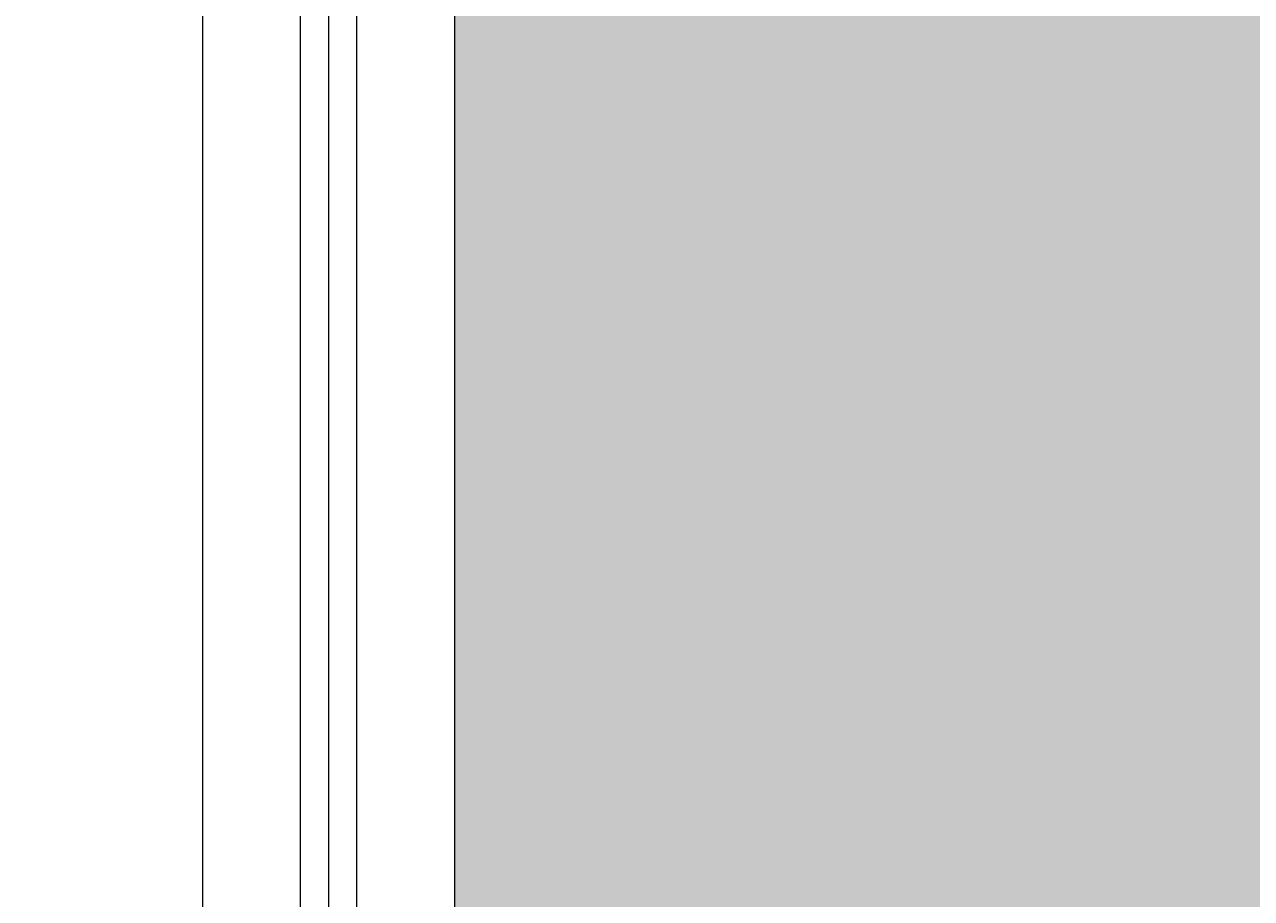
# Model space of a CAD drawing. Units: inches. Extents: x 84 to 1044, y -280 to 906.
# Tile 73 of 105: x 689 to 733, y 450 to 481. Entities that reach past the tile are written whole.
import ezdxf

# ---------------------------------------------------------------- set-up
doc = ezdxf.new("R2010")
doc.units = ezdxf.units.IN
doc.layers.add('A-ANNO-DIMS', color=2, linetype='Continuous', lineweight=18)
doc.layers.add('WINDOW', color=160, linetype='Continuous', lineweight=13)
doc.layers.add('L-PLNT-PATT', color=9, linetype='Continuous', lineweight=9, true_color=0xafd9aa)
doc.styles.get("Standard").update_dxf_attribs({"font": 'arial.ttf'})
doc.dimstyles.get("Standard").update_dxf_attribs({"dimtxt": 0.18, "dimasz": 0.18, "dimexe": 0.18, "dimexo": 0.0625, "dimgap": 0.09, "dimtad": 0, "dimtih": 1, "dimtoh": 1, "dimdec": 4, "dimzin": 0, "dimdsep": 46, "dimtxsty": 'Standard', "dimcen": 0.09, "dimadec": 0, "dimazin": 0, "dimtfac": 1, "dimtdec": 4, "dimtofl": 0, "dimtmove": 0, "dimatfit": 3, "dimfxl": 1, "dimtolj": 1, "dimtzin": 0, "dimarcsym": 0})

# ---------------------------------------------------------------- blocks, each defined once
blk = doc.blocks.new('WIN-72IN')
for p, q in [((72.004, 9), (0.004, 9)), ((72.004, 5.5), (0.004, 5.5)), ((72.004, 4.5), (0.004, 4.5)), ((72.004, 3.5), (0.004, 3.5)), ((0.004, 0), (72.004, 0))]:
    blk.add_line(p, q)
blk = doc.blocks.new('*D62')
at = {"layer": 'A-ANNO-DIMS', "color": 0, "lineweight": -2, "transparency": 16777216}
for p, q in [((203.179, 709.183), (203.179, 905.9)), ((896.074, 400.183), (896.074, 905.9)), ((203.359, 905.72), (549.232, 905.72)), ((895.894, 905.72), (550.021, 905.72))]:
    blk.add_line(p, q, dxfattribs=at)
at = {"layer": 'A-ANNO-DIMS', "color": 0, "transparency": 16777216}
for points in [[(203.359, 905.75), (203.359, 905.69), (203.179, 905.72)], [(895.894, 905.75), (895.894, 905.69), (896.074, 905.72)]]:
    blk.add_solid(points, dxfattribs=at)
at = {"layer": 'Defpoints', "color": 0, "transparency": 16777216}
for p in [(896.074, 905.72), (203.179, 709.12), (896.074, 400.12)]:
    blk.add_point(p, dxfattribs=at)
at = {"layer": 'A-ANNO-DIMS', "color": 0, "transparency": 16777216, "insert": (549.627, 905.72), "char_height": 0.18, "attachment_point": 5}
blk.add_mtext('\\A1;692.9', dxfattribs=at)

msp = doc.modelspace()

# ---------------------------------------------------------------- hatches: boundary and pattern name
at = {"layer": 'L-PLNT-PATT', "transparency": 33554597}
h = msp.add_hatch(color=256, dxfattribs=at)
h.dxf.hatch_style = 1
h.paths.add_polyline_path([(896.074, 511.12), (704.074, 511.12), (704.074, 491.62), (704.074, 419.62), (704.074, 400.12), (833.074, 400.12), (896.074, 400.12)])

# ---------------------------------------------------------------- block references
at = {"layer": 'WINDOW', "rotation": 270.0000000000001}
msp.add_blockref('WIN-72IN', (695.074, 491.624), dxfattribs=at)

# ---------------------------------------------------------------- dimensions: what is measured, and where the dimension line sits
at = {"layer": 'A-ANNO-DIMS'}
dim = msp.add_linear_dim(base=(896.074, 905.72), p1=(203.179, 709.12), p2=(896.074, 400.12), dimstyle='Standard', override={"dimdec": 1, "dimlfac": 1, "dimrnd": 0, "dimzin": 0, "dimdsep": 46, "dimlunit": 2}, dxfattribs=at)
dim.commit()
dim.dimension.update_dxf_attribs({"geometry": '*D62', "text_midpoint": (549.627, 905.72)})

doc.saveas('drawing.dxf')
